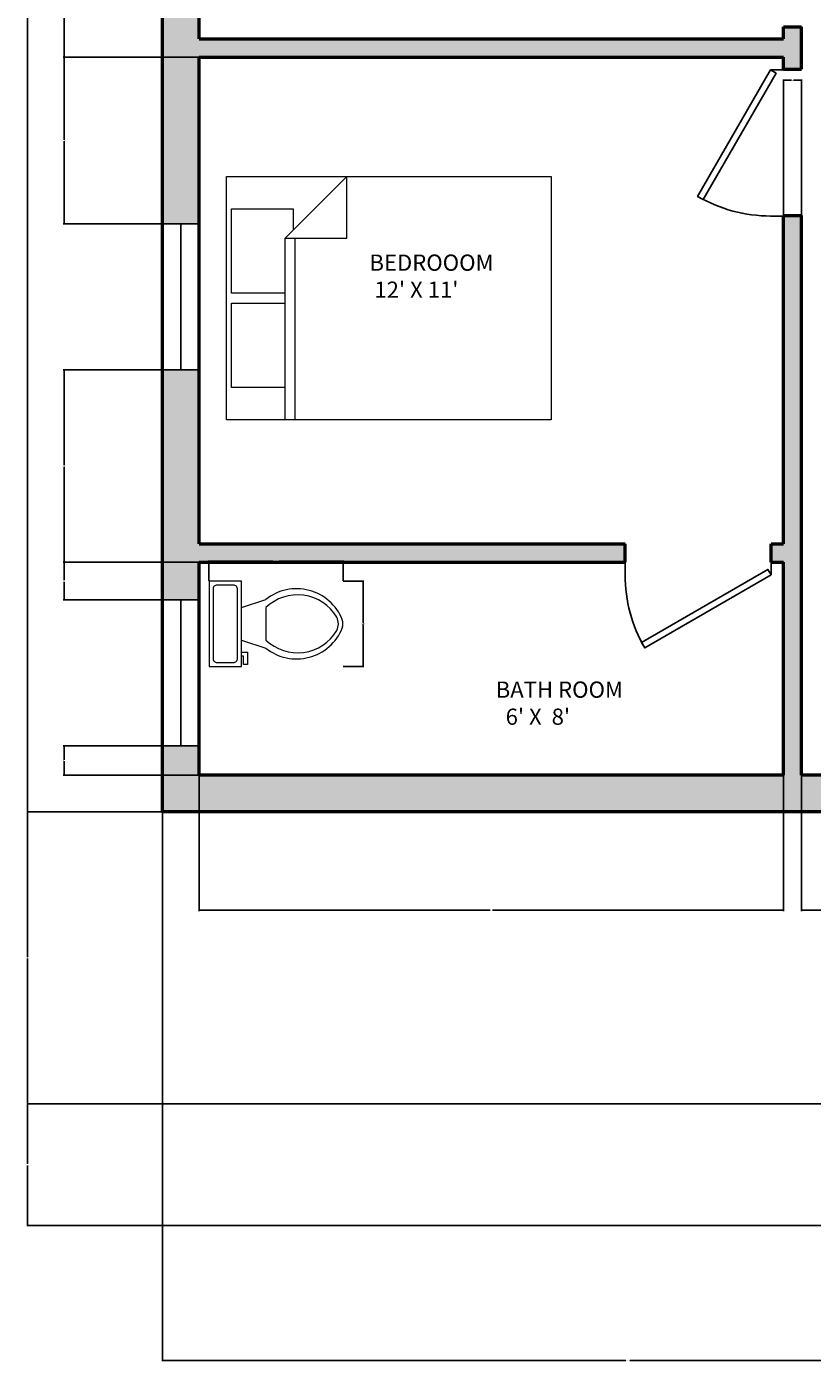
# Model space of a CAD drawing. Units: inches. Extents: x 4 to 671, y -79 to 570.
# Tile 1 of 7: x 4 to 198, y -79 to 250. Entities that reach past the tile are written whole.
import ezdxf

# ---------------------------------------------------------------- set-up
doc = ezdxf.new("R2010")
doc.units = ezdxf.units.IN
doc.header["$MEASUREMENT"] = 0
for name, color, linetype, lineweight in [('A-ANNO-DIMS', 2, 'Continuous', 18), ('A-AREA-IDEN', 7, 'Continuous', 18), ('A-WALL', 7, 'Continuous', 50), ('A-WALL-PATT', 251, 'Continuous', 13), ('bathroom', 90, 'Continuous', 18), ('doors', 40, 'Continuous', 25), ('furniture', 220, 'Continuous', 18), ('window', 30, 'Continuous', 25)]:
    doc.layers.add(name, color=color, linetype=linetype, lineweight=lineweight)
doc.styles.get("Standard").update_dxf_attribs({"font": 'arial.ttf'})
doc.dimstyles.get("Standard").update_dxf_attribs({"dimtxt": 0.18, "dimasz": 0.18, "dimexe": 0.18, "dimexo": 0.0625, "dimgap": 0.09, "dimtad": 0, "dimtih": 1, "dimtoh": 1, "dimdec": 4, "dimzin": 0, "dimdsep": 46, "dimtxsty": 'Standard', "dimcen": 0.09, "dimadec": 0, "dimazin": 0, "dimtfac": 1, "dimtdec": 4, "dimtofl": 0, "dimtmove": 0, "dimatfit": 3, "dimfxl": 1, "dimtolj": 1, "dimtzin": 0, "dimarcsym": 0})

# ---------------------------------------------------------------- blocks, each defined once
blk = doc.blocks.new('*U9')
for p, q in [((0, 0), (0, -6)), ((40, 0), (40, -6))]:
    blk.add_line(p, q)
blk.add_lwpolyline([(0, 0), (34.64, 20), (35.52, 18.48), (0.87, -1.52)], close=True)
blk.add_arc((0, 0), 40, 0, 30)
blk = doc.blocks.new('Bed - Queen')
for p, q in [((0, -80.00003), (0, 0)), ((0, 0), (59.99999, 0)), ((59.99999, 0), (59.99999, -80.00003)), ((7.99999, -1.2), (28.79998, -1.2)), ((7.99999, -14.4), (7.99999, -1.2)), ((28.79998, -1.2), (28.79998, -14.4)), ((31.19999, -1.2), (51.99999, -1.2)), ((31.19999, -14.4), (31.19999, -1.2)), ((51.99999, -1.2), (51.99999, -16.4)), ((0, -14.4), (44.8, -14.4)), ((59.99999, -29.6), (44.8, -14.4)), ((44.8, -14.4), (44.8, -29.6)), ((51.99999, -16.4), (46.79936, -16.4)), ((44.8, -16.8), (0, -16.8)), ((44.8, -29.6), (59.99999, -29.6)), ((59.99999, -80.00003), (0, -80.00003))]:
    blk.add_line(p, q)
blk = doc.blocks.new('Toilet - top')
for p, q in [((9.5, -6), (9.5, -2)), ((-10, -8.5), (-8, -8.5)), ((-10, -9.5), (-10, -8.5)), ((-7, -9.5), (-10, -9.5)), ((-8, -8.5), (-8, -8)), ((-7, -8), (-7, -9.5)), ((-4, -8), (-6, -14)), ((4, -8), (6, -14)), ((4, -14), (-4, -14))]:
    blk.add_line(p, q)
blk.add_lwpolyline([(10.5, -8), (10.5, 0), (-10.5, 0), (-10.5, -8)], close=True)
for points in [[(-9.5, -2), (-9.5, -6)], [(8.5, -1), (-8.5, -1)], [(-8.5, -7), (8.5, -7)]]:
    blk.add_lwpolyline(points)
for centre, radius, start, end in [((-8.62, -1.88), 0.884, 81.8699, 188.1301), ((8.62, -1.88), 0.884, 351.8699, 98.1301), ((-8.62, -6.12), 0.884, 171.8699, 278.1301), ((8.62, -6.12), 0.884, 261.8699, 8.1301), ((3.52, -21.58), 12.17, 141.4691, 247.9714), ((4.2, -21.82), 11.33, 136.3677, 238.9468), ((-3.52, -21.58), 12.17, 292.0284, 38.5307), ((-4.2, -21.82), 11.33, 301.053, 43.6321), ((0, -27.88), 4, 245.7318, 294.2682), ((0, -29), 4, 254.8605, 285.1395)]:
    blk.add_arc(centre, radius, start, end)
blk = doc.blocks.new('*U12')
for p, q in [((0, 0), (0, -6)), ((-40, 0), (-40, -6))]:
    blk.add_line(p, q)
blk.add_lwpolyline([(0, 0), (-34.64, 20), (-35.52, 18.48), (-0.88, -1.52)], close=True)
blk.add_arc((0, 0), 40, 150, 180)
blk = doc.blocks.new('WIN-36')
for p, q in [((0, 0), (0, 9)), ((0, 9), (36, 9)), ((36, 9), (36, 0)), ((36, 9), (36, 4.5)), ((36, 4.5), (0, 4.5)), ((36, 0), (0, 0))]:
    blk.add_line(p, q)
blk = doc.blocks.new('*D29')
at = {"layer": 'A-ANNO-DIMS', "color": 0, "lineweight": -2, "transparency": 16777216}
for p, q in [((48.87, 113.22), (48.87, 118.3)), ((49.05, 118.12), (64.62, 118.12)), ((81.74, 118.12), (66.17, 118.12)), ((81.92, 113.22), (81.92, 118.3))]:
    blk.add_line(p, q, dxfattribs=at)
at = {"layer": 'A-ANNO-DIMS', "color": 0, "transparency": 16777216}
for points in [[(49.05, 118.15), (49.05, 118.09), (48.87, 118.12)], [(81.74, 118.15), (81.74, 118.09), (81.92, 118.12)]]:
    blk.add_solid(points, dxfattribs=at)
at = {"layer": 'Defpoints', "color": 0, "transparency": 16777216}
for p in [(48.87, 118.12), (48.87, 113.16), (81.92, 113.16)]:
    blk.add_point(p, dxfattribs=at)
at = {"layer": 'A-ANNO-DIMS', "color": 0, "transparency": 16777216, "insert": (65.4, 118.12), "char_height": 0.18, "attachment_point": 5}
blk.add_mtext('\\A1;WC 33 TYP.', dxfattribs=at)
blk = doc.blocks.new('*D30')
at = {"layer": 'A-ANNO-DIMS', "color": 0, "lineweight": -2, "transparency": 16777216}
for p, q in [((81.98, 113.16), (87.06, 113.16)), ((86.88, 112.98), (86.88, 102.84)), ((86.88, 92.34), (86.88, 102.48)), ((81.98, 92.16), (87.06, 92.16))]:
    blk.add_line(p, q, dxfattribs=at)
at = {"layer": 'A-ANNO-DIMS', "color": 0, "transparency": 16777216}
for points in [[(86.85, 112.98), (86.91, 112.98), (86.88, 113.16)], [(86.85, 92.34), (86.91, 92.34), (86.88, 92.16)]]:
    blk.add_solid(points, dxfattribs=at)
at = {"layer": 'Defpoints', "color": 0, "transparency": 16777216}
for p in [(81.92, 113.16), (86.88, 113.16), (81.92, 92.16)]:
    blk.add_point(p, dxfattribs=at)
at = {"layer": 'A-ANNO-DIMS', "color": 0, "transparency": 16777216, "insert": (86.88, 102.66), "char_height": 0.18, "attachment_point": 5}
blk.add_mtext('\\A1;21 TYP.', dxfattribs=at)
blk = doc.blocks.new('*D51')
at = {"layer": 'A-ANNO-DIMS', "color": 0, "lineweight": -2, "transparency": 16777216}
for p, q in [((37.38, 536.35), (3.96, 536.35)), ((4.14, 536.17), (4.14, 296.53)), ((4.14, 56.53), (4.14, 296.17)), ((37.38, 56.35), (3.96, 56.35))]:
    blk.add_line(p, q, dxfattribs=at)
at = {"layer": 'A-ANNO-DIMS', "color": 0, "transparency": 16777216}
for points in [[(4.11, 536.17), (4.17, 536.17), (4.14, 536.35)], [(4.11, 56.53), (4.17, 56.53), (4.14, 56.35)]]:
    blk.add_solid(points, dxfattribs=at)
at = {"layer": 'Defpoints', "color": 0, "transparency": 16777216}
for p in [(4.14, 536.35), (37.44, 536.35), (37.44, 56.35)]:
    blk.add_point(p, dxfattribs=at)
at = {"layer": 'A-ANNO-DIMS', "color": 0, "transparency": 16777216, "insert": (4.14, 296.35), "char_height": 0.18, "attachment_point": 5}
blk.add_mtext('\\A1;480', dxfattribs=at)
blk = doc.blocks.new('*D52')
at = {"layer": 'A-ANNO-DIMS', "color": 0, "lineweight": -2, "transparency": 16777216}
for p, q in [((37.38, 56.35), (3.96, 56.35)), ((4.14, 56.17), (4.14, 20.53)), ((4.14, -15.47), (4.14, 20.17)), ((266.74, -15.65), (3.96, -15.65))]:
    blk.add_line(p, q, dxfattribs=at)
at = {"layer": 'A-ANNO-DIMS', "color": 0, "transparency": 16777216}
for points in [[(4.11, 56.17), (4.17, 56.17), (4.14, 56.35)], [(4.11, -15.47), (4.17, -15.47), (4.14, -15.65)]]:
    blk.add_solid(points, dxfattribs=at)
at = {"layer": 'Defpoints', "color": 0, "transparency": 16777216}
for p in [(4.14, 56.35), (37.44, 56.35), (266.8, -15.65)]:
    blk.add_point(p, dxfattribs=at)
at = {"layer": 'A-ANNO-DIMS', "color": 0, "transparency": 16777216, "insert": (4.14, 20.35), "char_height": 0.18, "attachment_point": 5}
blk.add_mtext('\\A1;72', dxfattribs=at)
blk = doc.blocks.new('*D53')
at = {"layer": 'A-ANNO-DIMS', "color": 0, "lineweight": -2, "transparency": 16777216}
for p, q in [((266.74, -15.65), (3.96, -15.65)), ((4.14, -15.83), (4.14, -30.47)), ((4.14, -45.47), (4.14, -30.83)), ((283.74, -45.65), (3.96, -45.65))]:
    blk.add_line(p, q, dxfattribs=at)
at = {"layer": 'A-ANNO-DIMS', "color": 0, "transparency": 16777216}
for points in [[(4.11, -15.83), (4.17, -15.83), (4.14, -15.65)], [(4.11, -45.47), (4.17, -45.47), (4.14, -45.65)]]:
    blk.add_solid(points, dxfattribs=at)
at = {"layer": 'Defpoints', "color": 0, "transparency": 16777216}
for p in [(4.14, -15.65), (266.8, -15.65), (283.8, -45.65)]:
    blk.add_point(p, dxfattribs=at)
at = {"layer": 'A-ANNO-DIMS', "color": 0, "transparency": 16777216, "insert": (4.14, -30.65), "char_height": 0.18, "attachment_point": 5}
blk.add_mtext('\\A1;30', dxfattribs=at)
blk = doc.blocks.new('*D54')
at = {"layer": 'A-ANNO-DIMS', "color": 0, "lineweight": -2, "transparency": 16777216}
for p, q in [((37.44, 56.29), (37.44, -79.13)), ((266.8, -15.71), (266.8, -79.13)), ((37.62, -78.95), (151.65, -78.95)), ((266.62, -78.95), (152.59, -78.95))]:
    blk.add_line(p, q, dxfattribs=at)
at = {"layer": 'A-ANNO-DIMS', "color": 0, "transparency": 16777216}
for points in [[(37.62, -78.92), (37.62, -78.98), (37.44, -78.95)], [(266.62, -78.92), (266.62, -78.98), (266.8, -78.95)]]:
    blk.add_solid(points, dxfattribs=at)
at = {"layer": 'Defpoints', "color": 0, "transparency": 16777216}
for p in [(37.44, 56.35), (266.8, -15.65), (266.8, -78.95)]:
    blk.add_point(p, dxfattribs=at)
at = {"layer": 'A-ANNO-DIMS', "color": 0, "transparency": 16777216, "insert": (152.12, -78.95), "char_height": 0.18, "attachment_point": 5}
blk.add_mtext('\\A1;229.36', dxfattribs=at)
blk = doc.blocks.new('*D63')
at = {"layer": 'A-ANNO-DIMS', "color": 0, "lineweight": -2, "transparency": 16777216}
for p, q in [((46.44, 65.29), (46.44, 31.87)), ((190.44, 65.29), (190.44, 31.87)), ((46.62, 32.05), (118.16, 32.05)), ((190.26, 32.05), (118.72, 32.05))]:
    blk.add_line(p, q, dxfattribs=at)
at = {"layer": 'A-ANNO-DIMS', "color": 0, "transparency": 16777216}
for points in [[(46.62, 32.08), (46.62, 32.02), (46.44, 32.05)], [(190.26, 32.08), (190.26, 32.02), (190.44, 32.05)]]:
    blk.add_solid(points, dxfattribs=at)
at = {"layer": 'Defpoints', "color": 0, "transparency": 16777216}
for p in [(46.44, 65.35), (190.44, 65.35), (46.44, 32.05)]:
    blk.add_point(p, dxfattribs=at)
at = {"layer": 'A-ANNO-DIMS', "color": 0, "transparency": 16777216, "insert": (118.44, 32.05), "char_height": 0.18, "attachment_point": 5}
blk.add_mtext('\\A1;144', dxfattribs=at)
blk = doc.blocks.new('*D65')
at = {"layer": 'A-ANNO-DIMS', "color": 0, "lineweight": -2, "transparency": 16777216}
for p, q in [((46.38, 72.55), (12.96, 72.55)), ((13.14, 72.37), (13.14, 69.13)), ((13.14, 65.53), (13.14, 68.77)), ((46.38, 65.35), (12.96, 65.35))]:
    blk.add_line(p, q, dxfattribs=at)
at = {"layer": 'A-ANNO-DIMS', "color": 0, "transparency": 16777216}
for points in [[(13.11, 72.37), (13.17, 72.37), (13.14, 72.55)], [(13.11, 65.53), (13.17, 65.53), (13.14, 65.35)]]:
    blk.add_solid(points, dxfattribs=at)
at = {"layer": 'Defpoints', "color": 0, "transparency": 16777216}
for p in [(13.14, 72.55), (46.44, 72.55), (46.44, 65.35)]:
    blk.add_point(p, dxfattribs=at)
at = {"layer": 'A-ANNO-DIMS', "color": 0, "transparency": 16777216, "insert": (13.14, 68.95), "char_height": 0.18, "attachment_point": 5}
blk.add_mtext('\\A1;7.201', dxfattribs=at)
blk = doc.blocks.new('*D66')
at = {"layer": 'A-ANNO-DIMS', "color": 0, "lineweight": -2, "transparency": 16777216}
for p, q in [((46.38, 117.85), (12.96, 117.85)), ((13.14, 117.67), (13.14, 113.38)), ((13.14, 108.73), (13.14, 113.02)), ((46.38, 108.55), (12.96, 108.55))]:
    blk.add_line(p, q, dxfattribs=at)
at = {"layer": 'A-ANNO-DIMS', "color": 0, "transparency": 16777216}
for points in [[(13.11, 117.67), (13.17, 117.67), (13.14, 117.85)], [(13.11, 108.73), (13.17, 108.73), (13.14, 108.55)]]:
    blk.add_solid(points, dxfattribs=at)
at = {"layer": 'Defpoints', "color": 0, "transparency": 16777216}
for p in [(13.14, 117.85), (46.44, 117.85), (46.44, 108.55)]:
    blk.add_point(p, dxfattribs=at)
at = {"layer": 'A-ANNO-DIMS', "color": 0, "transparency": 16777216, "insert": (13.14, 113.2), "char_height": 0.18, "attachment_point": 5}
blk.add_mtext('\\A1;9.3', dxfattribs=at)
blk = doc.blocks.new('*D67')
at = {"layer": 'A-ANNO-DIMS', "color": 0, "lineweight": -2, "transparency": 16777216}
for p, q in [((46.38, 165.27), (12.96, 165.27)), ((13.14, 165.09), (13.14, 141.74)), ((13.14, 118.03), (13.14, 141.38)), ((46.38, 117.85), (12.96, 117.85))]:
    blk.add_line(p, q, dxfattribs=at)
at = {"layer": 'A-ANNO-DIMS', "color": 0, "transparency": 16777216}
for points in [[(13.11, 165.09), (13.17, 165.09), (13.14, 165.27)], [(13.11, 118.03), (13.17, 118.03), (13.14, 117.85)]]:
    blk.add_solid(points, dxfattribs=at)
at = {"layer": 'Defpoints', "color": 0, "transparency": 16777216}
for p in [(13.14, 165.27), (46.44, 165.27), (46.44, 117.85)]:
    blk.add_point(p, dxfattribs=at)
at = {"layer": 'A-ANNO-DIMS', "color": 0, "transparency": 16777216, "insert": (13.14, 141.56), "char_height": 0.18, "attachment_point": 5}
blk.add_mtext('\\A1;47.415', dxfattribs=at)
blk = doc.blocks.new('*D68')
at = {"layer": 'A-ANNO-DIMS', "color": 0, "lineweight": -2, "transparency": 16777216}
for p, q in [((46.38, 242.35), (12.96, 242.35)), ((13.14, 242.17), (13.14, 221.99)), ((13.14, 201.45), (13.14, 221.63)), ((46.38, 201.27), (12.96, 201.27))]:
    blk.add_line(p, q, dxfattribs=at)
at = {"layer": 'A-ANNO-DIMS', "color": 0, "transparency": 16777216}
for points in [[(13.11, 242.17), (13.17, 242.17), (13.14, 242.35)], [(13.11, 201.45), (13.17, 201.45), (13.14, 201.27)]]:
    blk.add_solid(points, dxfattribs=at)
at = {"layer": 'Defpoints', "color": 0, "transparency": 16777216}
for p in [(13.14, 242.35), (46.44, 242.35), (46.44, 201.27)]:
    blk.add_point(p, dxfattribs=at)
at = {"layer": 'A-ANNO-DIMS', "color": 0, "transparency": 16777216, "insert": (13.14, 221.81), "char_height": 0.18, "attachment_point": 5}
blk.add_mtext('\\A1;41.085', dxfattribs=at)
blk = doc.blocks.new('*D69')
at = {"layer": 'A-ANNO-DIMS', "color": 0, "lineweight": -2, "transparency": 16777216}
for p, q in [((46.38, 303.54), (12.96, 303.54)), ((13.14, 303.36), (13.14, 273.13)), ((13.14, 242.53), (13.14, 272.76)), ((46.38, 242.35), (12.96, 242.35))]:
    blk.add_line(p, q, dxfattribs=at)
at = {"layer": 'A-ANNO-DIMS', "color": 0, "transparency": 16777216}
for points in [[(13.11, 303.36), (13.17, 303.36), (13.14, 303.54)], [(13.11, 242.53), (13.17, 242.53), (13.14, 242.35)]]:
    blk.add_solid(points, dxfattribs=at)
at = {"layer": 'Defpoints', "color": 0, "transparency": 16777216}
for p in [(13.14, 303.54), (46.44, 303.54), (46.44, 242.35)]:
    blk.add_point(p, dxfattribs=at)
at = {"layer": 'A-ANNO-DIMS', "color": 0, "transparency": 16777216, "insert": (13.14, 272.94), "char_height": 0.18, "attachment_point": 5}
blk.add_mtext('\\A1;61.19', dxfattribs=at)
blk = doc.blocks.new('*D85')
at = {"layer": 'A-ANNO-DIMS', "color": 0, "lineweight": -2, "transparency": 16777216}
for p, q in [((194.94, 65.29), (194.94, 31.87)), ((218.8, 65.29), (218.8, 31.87)), ((195.12, 32.05), (206.47, 32.05)), ((218.62, 32.05), (207.27, 32.05))]:
    blk.add_line(p, q, dxfattribs=at)
at = {"layer": 'A-ANNO-DIMS', "color": 0, "transparency": 16777216}
for points in [[(195.12, 32.08), (195.12, 32.02), (194.94, 32.05)], [(218.62, 32.08), (218.62, 32.02), (218.8, 32.05)]]:
    blk.add_solid(points, dxfattribs=at)
at = {"layer": 'Defpoints', "color": 0, "transparency": 16777216}
for p in [(194.94, 65.35), (218.8, 65.35), (194.94, 32.05)]:
    blk.add_point(p, dxfattribs=at)
at = {"layer": 'A-ANNO-DIMS', "color": 0, "transparency": 16777216, "insert": (206.87, 32.05), "char_height": 0.18, "attachment_point": 5}
blk.add_mtext('\\A1;23.86', dxfattribs=at)
blk = doc.blocks.new('*D97')
at = {"layer": 'A-ANNO-DIMS', "color": 0, "lineweight": -2, "transparency": 16777216}
for p, q in [((190.44, 203.41), (190.44, 236.83)), ((190.62, 236.65), (192.43, 236.65)), ((194.76, 236.65), (192.95, 236.65)), ((194.94, 203.41), (194.94, 236.83))]:
    blk.add_line(p, q, dxfattribs=at)
at = {"layer": 'A-ANNO-DIMS', "color": 0, "transparency": 16777216}
for points in [[(190.62, 236.68), (190.62, 236.62), (190.44, 236.65)], [(194.76, 236.68), (194.76, 236.62), (194.94, 236.65)]]:
    blk.add_solid(points, dxfattribs=at)
at = {"layer": 'Defpoints', "color": 0, "transparency": 16777216}
for p in [(194.94, 236.65), (190.44, 203.35), (194.94, 203.35)]:
    blk.add_point(p, dxfattribs=at)
at = {"layer": 'A-ANNO-DIMS', "color": 0, "transparency": 16777216, "insert": (192.69, 236.65), "char_height": 0.18, "attachment_point": 5}
blk.add_mtext('\\A1;4.5', dxfattribs=at)

msp = doc.modelspace()

# ---------------------------------------------------------------- hatches: boundary and pattern name
at = {"layer": 'A-WALL-PATT'}
h = msp.add_hatch(color=256, dxfattribs=at)
h.dxf.hatch_style = 1
h.paths.add_polyline_path([(46.4392, 165.2664), (37.4392, 165.2664), (37.4392, 108.5522), (41.9392, 108.5522), (46.4392, 108.5522), (46.4392, 117.8513), (151.434, 117.8513), (151.434, 120.1013), (151.434, 122.3513), (46.4392, 122.3513)], flags=17)
h.paths.add_polyline_path([(194.9392, 203.3513), (190.4392, 203.3513), (190.4392, 122.3513), (187.434, 122.3513), (187.434, 117.8513), (190.4392, 117.8513), (190.4392, 65.3513), (46.4392, 65.3513), (46.4392, 72.5522), (37.4392, 72.5522), (37.4392, 56.3513), (218.8007, 56.3513), (218.8007, 65.3513), (194.9392, 65.3513)])
h.paths.add_polyline_path([(46.4392, 242.3513), (190.4392, 242.3513), (190.4392, 239.3513), (194.9392, 239.3513), (194.9392, 249.8513), (190.4392, 249.8513), (190.4392, 246.8513), (46.4392, 246.8513), (46.4392, 303.5372), (37.4392, 303.5372), (37.4392, 201.2664), (41.9392, 201.2664), (46.4392, 201.2664)])
h.paths.add_polyline_path([(46.4392, 378.8513), (190.4392, 378.8513), (190.4392, 285.8513), (194.9392, 285.8513), (194.9392, 378.8513), (295.4392, 378.8513), (295.4392, 386.3513), (290.9392, 386.3513), (290.9392, 383.3513), (122.9392, 383.3513), (122.9392, 386.3513), (118.4392, 386.3513), (118.4392, 383.3513), (46.4392, 383.3513), (46.4392, 438.8513), (79.4392, 438.8513), (79.4392, 443.3513), (46.4392, 443.3513), (46.4392, 527.3513), (57.0095, 527.3513), (57.0095, 536.3513), (37.4392, 536.3513), (37.4392, 339.5372), (41.9392, 339.5372), (46.4392, 339.5372)])

# ---------------------------------------------------------------- linework, layer by layer
at = {"layer": 'A-WALL'}
for p, q in [((46.4392, 246.8513), (46.4392, 378.8513)), ((46.4392, 246.8513), (190.4392, 246.8513)), ((190.4392, 249.8513), (194.9392, 249.8513)), ((190.4392, 246.8513), (190.4392, 249.8513)), ((194.9392, 239.3513), (194.9392, 249.8513)), ((46.4392, 242.3513), (190.4392, 242.3513)), ((46.4392, 122.3513), (46.4392, 242.3513)), ((190.4392, 239.3513), (190.4392, 242.3513)), ((190.4392, 239.3513), (194.9392, 239.3513)), ((190.4392, 203.3513), (194.9392, 203.3513)), ((190.4392, 122.3513), (190.4392, 203.3513)), ((194.9392, 65.3513), (194.9392, 203.3513)), ((46.4392, 122.3513), (151.434, 122.3513)), ((151.434, 117.8513), (151.434, 122.3513)), ((187.434, 122.3513), (190.4392, 122.3513)), ((187.434, 117.8513), (187.434, 122.3513)), ((46.4392, 117.8513), (151.434, 117.8513)), ((46.4392, 65.3513), (46.4392, 117.8513)), ((187.434, 117.8513), (190.4392, 117.8513)), ((190.4392, 65.3513), (190.4392, 117.8513)), ((190.4392, 65.3513), (46.4392, 65.3513)), ((313.4392, 65.3513), (194.9392, 65.3513))]:
    msp.add_line(p, q, dxfattribs=at)
msp.add_lwpolyline([(313.4392, 56.3513), (37.4392, 56.3513), (37.4392, 536.3513), (637.4392, 536.3513), (637.4392, 56.3513), (362.9392, 56.3513)], dxfattribs=at)

# ---------------------------------------------------------------- block references
at = {"layer": 'bathroom', "rotation": 90}
msp.add_blockref('Toilet - top', (48.8722, 102.6593), dxfattribs=at)
at = {"layer": 'doors', "xscale": 0.9, "yscale": 0.9, "zscale": 0.9}
for name, p, rotation in [('*U12', (187.2975, 239.1872), 89.99999999995367), ('*U9', (187.434, 114.7013), 180)]:
    msp.add_blockref(name, p, dxfattribs=dict(at, rotation=rotation))
at = {"layer": 'furniture', "rotation": 90}
msp.add_blockref('Bed - Queen', (53.2164, 152.9288), dxfattribs=at)
at = {"layer": 'window'}
for p, rotation in [((46.4396, 165.266), 89.9999999999958), ((46.4396, 72.5519), 89.99999999999574)]:
    msp.add_blockref('WIN-36', p, dxfattribs=dict(at, rotation=rotation))

# ---------------------------------------------------------------- texts
at = {"layer": 'A-AREA-IDEN', "char_height": 4, "attachment_point": 1}
for s, insert in [("BEDROOOM\\P 12' X 11'", (88.4099, 193.6855)), ("BATH ROOM\\P  6' X  8'", (119.542, 88.4374))]:
    msp.add_mtext_dynamic_manual_height_columns(s, width=44.806469, gutter_width=1, heights=[0], dxfattribs=dict(at, insert=insert))

# ---------------------------------------------------------------- dimensions: what is measured, and where the dimension line sits
at = {"layer": 'A-ANNO-DIMS'}
for base, p1, p2, angle, override, picture, middle in [((4.1392, 536.3513), (37.4392, 56.3513), (37.4392, 536.3513), 90, {"dimdec": 0, "dimlfac": 1, "dimrnd": 0, "dimzin": 0, "dimdsep": 46, "dimlunit": 2}, '*D51', (4.1392, 296.3513)), ((13.1392, 303.5372), (46.4392, 242.3513), (46.4392, 303.5372), 90, {"dimdec": 2, "dimlfac": 1, "dimrnd": 0, "dimzin": 0, "dimdsep": 46, "dimlunit": 2}, '*D69', (13.1392, 272.9442)), ((13.1392, 242.3513), (46.4392, 201.2664), (46.4392, 242.3513), 90, {"dimdec": 3, "dimlfac": 1, "dimrnd": 0, "dimzin": 0, "dimdsep": 46, "dimlunit": 2}, '*D68', (13.1392, 221.8089)), ((13.1392, 165.2664), (46.4392, 117.8513), (46.4392, 165.2664), 90, {"dimdec": 3, "dimlfac": 1, "dimrnd": 0, "dimzin": 0, "dimdsep": 46, "dimlunit": 2}, '*D67', (13.1392, 141.5589)), ((13.1392, 117.8513), (46.4392, 108.5522), (46.4392, 117.8513), 90, {"dimdec": 1, "dimlfac": 1, "dimrnd": 0, "dimzin": 0, "dimdsep": 46, "dimlunit": 2}, '*D66', (13.1392, 113.2018)), ((13.1392, 72.5522), (46.4392, 65.3513), (46.4392, 72.5522), 90, {"dimdec": 3, "dimlfac": 1, "dimrnd": 0, "dimzin": 0, "dimdsep": 46, "dimlunit": 2}, '*D65', (13.1392, 68.9518)), ((46.4392, 32.0513), (190.4392, 65.3513), (46.4392, 65.3513), 180, {"dimdec": 0, "dimlfac": 1, "dimrnd": 0, "dimzin": 0, "dimdsep": 46, "dimlunit": 2}, '*D63', (118.4392, 32.0513)), ((194.9392, 32.0513), (218.8007, 65.3513), (194.9392, 65.3513), 180, {"dimdec": 2, "dimlfac": 1, "dimrnd": 0, "dimzin": 0, "dimdsep": 46, "dimlunit": 2}, '*D85', (206.87, 32.0513)), ((4.1392, 56.3513), (266.8007, -15.6487), (37.4392, 56.3513), 90, {"dimdec": 0, "dimlfac": 1, "dimrnd": 0, "dimzin": 0, "dimdsep": 46, "dimlunit": 2}, '*D52', (4.1392, 20.3513)), ((4.1392, -15.6487), (283.8007, -45.6487), (266.8007, -15.6487), 90, {"dimdec": 0, "dimlfac": 1, "dimrnd": 0, "dimzin": 0, "dimdsep": 46, "dimlunit": 2}, '*D53', (4.1392, -30.6487))]:
    dim = msp.add_linear_dim(base=base, p1=p1, p2=p2, angle=angle, dimstyle='Standard', override=override, dxfattribs=at)
    dim.commit()
    dim.dimension.update_dxf_attribs({"geometry": picture, "text_midpoint": middle})
for base, p1, p2, override, picture, middle in [((194.9392, 236.6513), (190.4392, 203.3513), (194.9392, 203.3513), {"dimdec": 1, "dimlfac": 1, "dimrnd": 0, "dimzin": 0, "dimdsep": 46, "dimlunit": 2}, '*D97', (192.6892, 236.6513)), ((266.8007, -78.9487), (37.4392, 56.3513), (266.8007, -15.6487), {"dimdec": 2, "dimlfac": 1, "dimrnd": 0, "dimzin": 0, "dimdsep": 46, "dimlunit": 2}, '*D54', (152.12, -78.9487))]:
    dim = msp.add_linear_dim(base=base, p1=p1, p2=p2, dimstyle='Standard', override=override, dxfattribs=at)
    dim.commit()
    dim.dimension.update_dxf_attribs({"geometry": picture, "text_midpoint": middle})
for base, p1, p2, angle, text, picture, middle in [((48.8722, 118.1163), (81.9185, 113.1593), (48.8722, 113.1593), 180, 'WC <> TYP.', '*D29', (65.3954, 118.1163)), ((86.8754, 113.1593), (81.9185, 92.1593), (81.9185, 113.1593), 90, '<> TYP.', '*D30', (86.8754, 102.6593))]:
    dim = msp.add_linear_dim(base=base, p1=p1, p2=p2, angle=angle, text=text, dimstyle='Standard', override={"dimdec": 0, "dimlfac": 1, "dimrnd": 0, "dimzin": 0, "dimdsep": 46, "dimlunit": 2}, dxfattribs=at)
    dim.commit()
    dim.dimension.update_dxf_attribs({"geometry": picture, "text_midpoint": middle})

doc.saveas('drawing.dxf')
